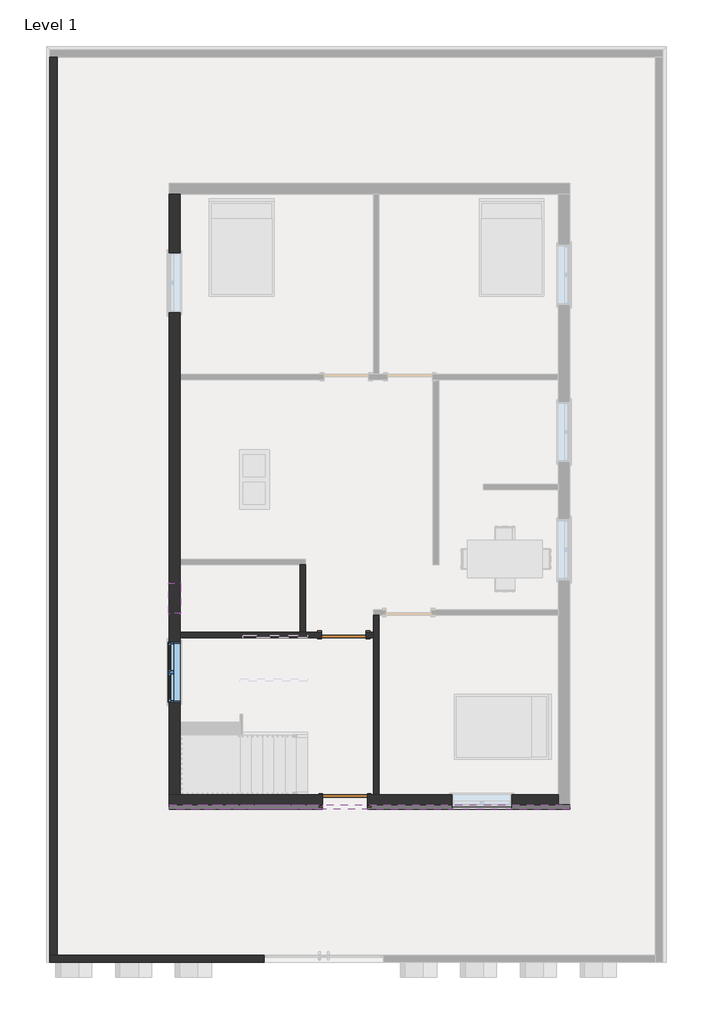
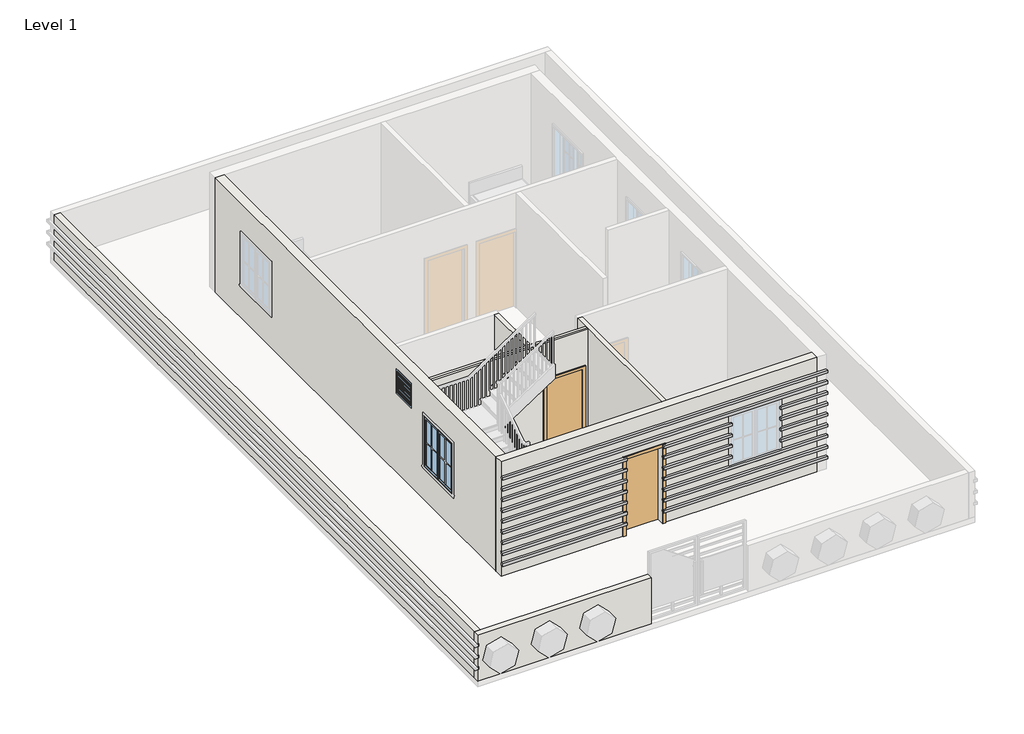
# One storey, part 1 of 4: 9 proxies, 7 walls, 2 doors, 2 windows.
"""IFC4 building model written with IfcOpenShell, lengths in millimetres."""

from ifc_helpers import new_model, si_unit, frame, origin, origin_with_axes, place, context, project, spatial, polyline, outline, extrude, faceted_brep, transform, mapped, element, save
from components import single_flush_door_3_5e62189b, single_flush_door_3_89fc3733, window_casement_double_window_4_576b2d2c, window_f2d8fef0

model = new_model("IFC4")

# Units and contexts
model_context = context("Model", 3, world=origin())
ifc_project = project(units=[si_unit("LENGTHUNIT", "METRE", prefix="MILLI")], contexts=[model_context])

# Site, building, storey
site = spatial("IfcSite", under=ifc_project)
building = spatial("IfcBuilding", under=site)
storey = spatial("IfcBuildingStorey", under=building, Name="Level 1", Elevation=0.0)

# Proxies
placement = place(None, origin())
element("IfcBuildingElementProxy", 1, Name="Reveal", ObjectType="Reveal", at=placement, inside=storey, context=model_context, shape_type="SweptSolid", body=[
    extrude(outline(polyline([(2831.4882597, -6585.4426559), (2831.4882597, -6677.5176559), (-1289.6617403, -6677.5176559), (-1289.6617403, -6585.4426559), (2831.4882597, -6585.4426559)])), frame((0.0, 0.0, 304.8), z_axis=(0.0, 0.0, 1.0), x_axis=(1.0, 0.0, 0.0)), (0.0, 0.0, 1.0), 67.7333333),
    extrude(outline(polyline([(-2204.0617403, -6585.4426559), (-2204.0617403, -6677.5176559), (-5334.6117403, -6677.5176559), (-5334.6117403, -6585.4426559), (-2204.0617403, -6585.4426559)])), frame((0.0, 0.0, 304.8), z_axis=(0.0, 0.0, 1.0), x_axis=(1.0, 0.0, 0.0)), (0.0, 0.0, 1.0), 67.7333333),
])
element("IfcBuildingElementProxy", 2, Name="Reveal", ObjectType="Reveal", at=placement, inside=storey, context=model_context, shape_type="SweptSolid", body=[
    extrude(outline(polyline([(2831.4882597, -6585.4426559), (2831.4882597, -6677.5176559), (-1289.6617403, -6677.5176559), (-1289.6617403, -6585.4426559), (2831.4882597, -6585.4426559)])), frame((0.0, 0.0, 591.2994231), z_axis=(0.0, 0.0, 1.0), x_axis=(1.0, 0.0, 0.0)), (0.0, 0.0, 1.0), 67.7333333),
    extrude(outline(polyline([(-2204.0617403, -6585.4426559), (-2204.0617403, -6677.5176559), (-5334.6117403, -6677.5176559), (-5334.6117403, -6585.4426559), (-2204.0617403, -6585.4426559)])), frame((0.0, 0.0, 591.2994231), z_axis=(0.0, 0.0, 1.0), x_axis=(1.0, 0.0, 0.0)), (0.0, 0.0, 1.0), 67.7333333),
])
element("IfcBuildingElementProxy", 3, Name="Reveal", ObjectType="Reveal", at=placement, inside=storey, context=model_context, shape_type="SweptSolid", body=[
    extrude(outline(polyline([(2831.4882597, -6585.4426559), (2831.4882597, -6677.5176559), (-1289.6617403, -6677.5176559), (-1289.6617403, -6585.4426559), (2831.4882597, -6585.4426559)])), frame((0.0, 0.0, 877.7988461), z_axis=(0.0, 0.0, 1.0), x_axis=(1.0, 0.0, 0.0)), (0.0, 0.0, 1.0), 67.7333333),
    extrude(outline(polyline([(-2204.0617403, -6585.4426559), (-2204.0617403, -6677.5176559), (-5334.6117403, -6677.5176559), (-5334.6117403, -6585.4426559), (-2204.0617403, -6585.4426559)])), frame((0.0, 0.0, 877.7988461), z_axis=(0.0, 0.0, 1.0), x_axis=(1.0, 0.0, 0.0)), (0.0, 0.0, 1.0), 67.7333333),
])
element("IfcBuildingElementProxy", 4, Name="Reveal", ObjectType="Reveal", at=placement, inside=storey, context=model_context, shape_type="SweptSolid", body=[
    extrude(outline(polyline([(2831.4882597, -6585.4426559), (2831.4882597, -6677.5176559), (1650.3882597, -6677.5176559), (1650.3882597, -6585.4426559), (2831.4882597, -6585.4426559)])), frame((0.0, 0.0, 1164.2982692), z_axis=(0.0, 0.0, 1.0), x_axis=(1.0, 0.0, 0.0)), (0.0, 0.0, 1.0), 67.7333333),
    extrude(outline(polyline([(431.1882597, -6585.4426559), (431.1882597, -6677.5176559), (-1289.6617403, -6677.5176559), (-1289.6617403, -6585.4426559), (431.1882597, -6585.4426559)])), frame((0.0, 0.0, 1164.2982692), z_axis=(0.0, 0.0, 1.0), x_axis=(1.0, 0.0, 0.0)), (0.0, 0.0, 1.0), 67.7333333),
    extrude(outline(polyline([(-2204.0617403, -6585.4426559), (-2204.0617403, -6677.5176559), (-5334.6117403, -6677.5176559), (-5334.6117403, -6585.4426559), (-2204.0617403, -6585.4426559)])), frame((0.0, 0.0, 1164.2982692), z_axis=(0.0, 0.0, 1.0), x_axis=(1.0, 0.0, 0.0)), (0.0, 0.0, 1.0), 67.7333333),
])
element("IfcBuildingElementProxy", 5, Name="Reveal", ObjectType="Reveal", at=placement, inside=storey, context=model_context, shape_type="SweptSolid", body=[
    extrude(outline(polyline([(2831.4882597, -6585.4426559), (2831.4882597, -6677.5176559), (1650.3882597, -6677.5176559), (1650.3882597, -6585.4426559), (2831.4882597, -6585.4426559)])), frame((0.0, 0.0, 1450.7976923), z_axis=(0.0, 0.0, 1.0), x_axis=(1.0, 0.0, 0.0)), (0.0, 0.0, 1.0), 67.7333333),
    extrude(outline(polyline([(431.1882597, -6585.4426559), (431.1882597, -6677.5176559), (-1289.6617403, -6677.5176559), (-1289.6617403, -6585.4426559), (431.1882597, -6585.4426559)])), frame((0.0, 0.0, 1450.7976923), z_axis=(0.0, 0.0, 1.0), x_axis=(1.0, 0.0, 0.0)), (0.0, 0.0, 1.0), 67.7333333),
    extrude(outline(polyline([(-2204.0617403, -6585.4426559), (-2204.0617403, -6677.5176559), (-5334.6117403, -6677.5176559), (-5334.6117403, -6585.4426559), (-2204.0617403, -6585.4426559)])), frame((0.0, 0.0, 1450.7976923), z_axis=(0.0, 0.0, 1.0), x_axis=(1.0, 0.0, 0.0)), (0.0, 0.0, 1.0), 67.7333333),
])
element("IfcBuildingElementProxy", 6, Name="Reveal", ObjectType="Reveal", at=placement, inside=storey, context=model_context, shape_type="SweptSolid", body=[
    extrude(outline(polyline([(2831.4882597, -6585.4426559), (2831.4882597, -6677.5176559), (1650.3882597, -6677.5176559), (1650.3882597, -6585.4426559), (2831.4882597, -6585.4426559)])), frame((0.0, 0.0, 1737.2971154), z_axis=(0.0, 0.0, 1.0), x_axis=(1.0, 0.0, 0.0)), (0.0, 0.0, 1.0), 67.7333333),
    extrude(outline(polyline([(431.1882597, -6585.4426559), (431.1882597, -6677.5176559), (-1289.6617403, -6677.5176559), (-1289.6617403, -6585.4426559), (431.1882597, -6585.4426559)])), frame((0.0, 0.0, 1737.2971154), z_axis=(0.0, 0.0, 1.0), x_axis=(1.0, 0.0, 0.0)), (0.0, 0.0, 1.0), 67.7333333),
    extrude(outline(polyline([(-2204.0617403, -6585.4426559), (-2204.0617403, -6677.5176559), (-5334.6117403, -6677.5176559), (-5334.6117403, -6585.4426559), (-2204.0617403, -6585.4426559)])), frame((0.0, 0.0, 1737.2971154), z_axis=(0.0, 0.0, 1.0), x_axis=(1.0, 0.0, 0.0)), (0.0, 0.0, 1.0), 67.7333333),
])
element("IfcBuildingElementProxy", 7, Name="Reveal", ObjectType="Reveal", at=placement, inside=storey, context=model_context, shape_type="SweptSolid", body=[
    extrude(outline(polyline([(2831.4882597, -6585.4426559), (2831.4882597, -6677.5176559), (1650.3882597, -6677.5176559), (1650.3882597, -6585.4426559), (2831.4882597, -6585.4426559)])), frame((0.0, 0.0, 2023.7965384), z_axis=(0.0, 0.0, 1.0), x_axis=(1.0, 0.0, 0.0)), (0.0, 0.0, 1.0), 67.7333333),
    extrude(outline(polyline([(431.1882597, -6585.4426559), (431.1882597, -6677.5176559), (-1289.6617403, -6677.5176559), (-1289.6617403, -6585.4426559), (431.1882597, -6585.4426559)])), frame((0.0, 0.0, 2023.7965384), z_axis=(0.0, 0.0, 1.0), x_axis=(1.0, 0.0, 0.0)), (0.0, 0.0, 1.0), 67.7333333),
    extrude(outline(polyline([(-2204.0617403, -6585.4426559), (-2204.0617403, -6677.5176559), (-5334.6117403, -6677.5176559), (-5334.6117403, -6585.4426559), (-2204.0617403, -6585.4426559)])), frame((0.0, 0.0, 2023.7965384), z_axis=(0.0, 0.0, 1.0), x_axis=(1.0, 0.0, 0.0)), (0.0, 0.0, 1.0), 67.7333333),
])
element("IfcBuildingElementProxy", 8, Name="Reveal", ObjectType="Reveal", at=placement, inside=storey, context=model_context, shape_type="SweptSolid", body=[
    extrude(outline(polyline([(2831.4882597, -6585.4426559), (2831.4882597, -6677.5176559), (-5334.6117403, -6677.5176559), (-5334.6117403, -6585.4426559), (2831.4882597, -6585.4426559)])), frame((0.0, 0.0, 2310.2959615), z_axis=(0.0, 0.0, 1.0), x_axis=(1.0, 0.0, 0.0)), (0.0, 0.0, 1.0), 67.7333333),
])
element("IfcBuildingElementProxy", 9, Name="Reveal", ObjectType="Reveal", at=placement, inside=storey, context=model_context, shape_type="SweptSolid", body=[
    extrude(outline(polyline([(2831.4882597, -6585.4426559), (2831.4882597, -6677.5176559), (-5334.6117403, -6677.5176559), (-5334.6117403, -6585.4426559), (2831.4882597, -6585.4426559)])), frame((0.0, 0.0, 2596.7953846), z_axis=(0.0, 0.0, 1.0), x_axis=(1.0, 0.0, 0.0)), (0.0, 0.0, 1.0), 67.7333333),
])

# Doors
single_flush_door_3_shape = single_flush_door_3_5e62189b(model_context)
element("IfcDoor", 10, ObjectType="Single-Flush : DOOR 3'", at=placement, inside=storey, context=model_context, shape_type="MappedRepresentation", body=[
    mapped(single_flush_door_3_shape, transform((-1772.2617403, -3124.6926559, 0.0), x_axis=(1.0, 0.0, 0.0), y_axis=(0.0, 1.0, 0.0), z_axis=(0.0, 0.0, 1.0))),
])
single_flush_door_3_2_shape = single_flush_door_3_89fc3733(model_context)
element("IfcDoor", 11, ObjectType="Single-Flush : DOOR 3'", at=placement, inside=storey, context=model_context, shape_type="MappedRepresentation", body=[
    mapped(single_flush_door_3_2_shape, transform((-1746.8617403, -6496.5426559, 0.0), x_axis=(1.0, 0.0, 0.0), y_axis=(0.0, 1.0, 0.0), z_axis=(0.0, 0.0, 1.0))),
])

# Walls
element("IfcWall", 12, ObjectType="ALL 4.5\"", at=placement, inside=storey, context=model_context, shape_type="Brep", body=[
    faceted_brep([(-1169.0117403, -2724.6426559, 0.0), (-1169.0117403, -3067.5426559, 0.0), (-1169.0117403, -3181.8426559, 0.0), (-1169.0117403, -6382.2426559, 0.0), (-1169.0117403, -6382.2426559, 3048.0), (-1169.0117403, -3181.8426559, 3048.0), (-1169.0117403, -3067.5426559, 3048.0), (-1169.0117403, -2724.6426559, 3048.0), (-1054.7117403, -2724.6426559, 0.0), (-1054.7117403, -2724.6426559, 3048.0), (-1054.7117403, -6382.2426559, 3048.0), (-1054.7117403, -6382.2426559, 0.0)], [[[0, 1, 2, 3, 4, 5, 6, 7]], [[8, 9, 10, 11]], [[3, 2, 1, 0, 8, 11]], [[0, 7, 9, 8]], [[4, 3, 11, 10]], [[7, 6, 5, 4, 10, 9]]]),
])
element("IfcWall", 13, ObjectType="ALL 4.5\"", at=placement, inside=storey, context=model_context, shape_type="Brep", body=[
    faceted_brep([(-1169.0117403, -3067.5426559, 0.0), (-1315.0617403, -3067.5426559, 0.0), (-1315.0617403, -3067.5426559, 2032.0), (-2229.4617403, -3067.5426559, 2032.0), (-2229.4617403, -3067.5426559, 0.0), (-2553.3117403, -3067.5426559, 0.0), (-2667.6117403, -3067.5426559, 0.0), (-5106.0117403, -3067.5426559, 0.0), (-5106.0117403, -3067.5426559, 3048.0), (-2667.6117403, -3067.5426559, 3048.0), (-2553.3117403, -3067.5426559, 3048.0), (-1169.0117403, -3067.5426559, 3048.0), (-1315.0617403, -3181.8426559, 2032.0), (-1315.0617403, -3181.8426559, 0.0), (-1169.0117403, -3181.8426559, 0.0), (-1169.0117403, -3181.8426559, 3048.0), (-5106.0117403, -3181.8426559, 3048.0), (-5106.0117403, -3181.8426559, 0.0), (-2229.4617403, -3181.8426559, 0.0), (-2229.4617403, -3181.8426559, 2032.0), (-5106.0117403, -3131.0426559, 3048.0), (-1169.0117403, -3131.0426559, 3048.0), (-2515.2117403, -3131.0426559, 3048.0)], [[[0, 1, 2, 3, 4, 5, 6, 7, 8, 9, 10, 11]], [[12, 13, 14, 15, 16, 17, 18, 19]], [[18, 17, 7, 6, 5, 4]], [[14, 13, 1, 0]], [[8, 7, 17, 16, 20]], [[0, 11, 21, 15, 14]], [[2, 1, 13, 12]], [[3, 2, 12, 19]], [[4, 3, 19, 18]], [[11, 10, 9, 8, 20, 22, 21]], [[20, 16, 15, 21, 22]]]),
])
element("IfcWall", 14, ObjectType="ALL 4.5\"", at=placement, inside=storey, context=model_context, shape_type="SweptSolid", body=[
    extrude(outline(polyline([(-2667.6117403, -3067.5426559), (-2667.6117403, -1695.9426559), (-2553.3117403, -1695.9426559), (-2553.3117403, -3067.5426559), (-2667.6117403, -3067.5426559)])), origin_with_axes(), (0.0, 0.0, 1.0), 3048.0),
])
element("IfcWall", 15, ObjectType="CMD 6\"", at=placement, inside=storey, context=model_context, shape_type="SweptSolid", body=[
    extrude(outline(polyline([(0.0, -7613.2753152), (1219.2, -7613.2753152), (1219.2, -7765.6753152), (982.1333333, -7765.6753152), (982.1333333, -7740.2753152), (914.4, -7740.2753152), (914.4, -7765.6753152), (677.3333333, -7765.6753152), (677.3333333, -7740.2753152), (609.6, -7740.2753152), (609.6, -7765.6753152), (372.5333333, -7765.6753152), (372.5333333, -7740.2753152), (304.8, -7740.2753152), (304.8, -7765.6753152), (0.0, -7765.6753152), (0.0, -7613.2753152)])), frame((0.0, -9645.3989753, 0.0), z_axis=(0.0, 1.0, 0.0), x_axis=(0.0, 0.0, 1.0)), (0.0, 0.0, 1.0), 18288.0),
])
element("IfcWall", 16, ObjectType="CMD 6\"", at=placement, inside=storey, context=model_context, shape_type="Brep", body=[
    faceted_brep([(-3397.8617403, -9645.3989753, 0.0), (-7613.2753152, -9645.3989753, 0.0), (-7765.6753152, -9645.3989753, 0.0), (-7765.6753152, -9645.3989753, 304.8), (-7740.2753152, -9645.3989753, 304.8), (-7740.2753152, -9645.3989753, 372.5333333), (-7765.6753152, -9645.3989753, 372.5333333), (-7765.6753152, -9645.3989753, 609.6), (-7740.2753152, -9645.3989753, 609.6), (-7740.2753152, -9645.3989753, 677.3333333), (-7765.6753152, -9645.3989753, 677.3333333), (-7765.6753152, -9645.3989753, 914.4), (-7740.2753152, -9645.3989753, 914.4), (-7740.2753152, -9645.3989753, 982.1333333), (-7765.6753152, -9645.3989753, 982.1333333), (-7765.6753152, -9645.3989753, 1219.2), (-7613.2753152, -9645.3989753, 1219.2), (-3397.8617403, -9645.3989753, 1219.2), (-7765.6753152, -9797.7989753, 0.0), (-3397.8617403, -9797.7989753, 0.0), (-3397.8617403, -9797.7989753, 1219.2), (-7765.6753152, -9797.7989753, 1219.2), (-7765.6753152, -9797.7989753, 982.1333333), (-7740.2753152, -9797.7989753, 982.1333333), (-7740.2753152, -9797.7989753, 914.4), (-7765.6753152, -9797.7989753, 914.4), (-7765.6753152, -9797.7989753, 677.3333333), (-7740.2753152, -9797.7989753, 677.3333333), (-7740.2753152, -9797.7989753, 609.6), (-7765.6753152, -9797.7989753, 609.6), (-7765.6753152, -9797.7989753, 372.5333333), (-7740.2753152, -9797.7989753, 372.5333333), (-7740.2753152, -9797.7989753, 304.8), (-7765.6753152, -9797.7989753, 304.8)], [[[0, 1, 2, 3, 4, 5, 6, 7, 8, 9, 10, 11, 12, 13, 14, 15, 16, 17]], [[18, 19, 20, 21, 22, 23, 24, 25, 26, 27, 28, 29, 30, 31, 32, 33]], [[2, 1, 0, 19, 18]], [[17, 16, 15, 21, 20]], [[0, 17, 20, 19]], [[2, 18, 33, 3]], [[21, 15, 14, 22]], [[6, 30, 29, 7]], [[10, 26, 25, 11]], [[5, 31, 30, 6]], [[32, 4, 3, 33]], [[31, 5, 4, 32]], [[9, 27, 26, 10]], [[28, 8, 7, 29]], [[27, 9, 8, 28]], [[13, 23, 22, 14]], [[24, 12, 11, 25]], [[23, 13, 12, 24]]]),
])
element("IfcWall", 17, ObjectType="WALL 9\"", at=placement, inside=storey, context=model_context, shape_type="Brep", body=[
    faceted_brep([(-5334.6117403, -6382.2426559, 3048.0), (-5106.0117403, -6382.2426559, 3048.0), (-1169.0117403, -6382.2426559, 3048.0), (-1054.7117403, -6382.2426559, 3048.0), (2602.8882597, -6382.2426559, 3048.0), (2602.8882597, -6382.2426559, 0.0), (-1054.7117403, -6382.2426559, 0.0), (-1169.0117403, -6382.2426559, 0.0), (-1289.6617403, -6382.2426559, 0.0), (-1289.6617403, -6382.2426559, 2032.0), (-2204.0617403, -6382.2426559, 2032.0), (-2204.0617403, -6382.2426559, 0.0), (-5106.0117403, -6382.2426559, 0.0), (-5334.6117403, -6382.2426559, 0.0), (431.1882597, -6382.2426559, 2260.6), (431.1882597, -6382.2426559, 914.4), (1650.3882597, -6382.2426559, 914.4), (1650.3882597, -6382.2426559, 2260.6), (2602.8882597, -6610.8426559, 3048.0), (-5334.6117403, -6610.8426559, 3048.0), (-5334.6117403, -6610.8426559, 2664.5287179), (2602.8882597, -6610.8426559, 2664.5287179), (431.1882597, -6610.8426559, 2260.6), (1650.3882597, -6610.8426559, 2260.6), (1650.3882597, -6610.8426559, 2091.5298718), (2602.8882597, -6610.8426559, 2091.5298718), (2602.8882597, -6610.8426559, 2310.2959615), (-5334.6117403, -6610.8426559, 2310.2959615), (-5334.6117403, -6610.8426559, 2091.5298718), (-2204.0617403, -6610.8426559, 2091.5298718), (-2204.0617403, -6610.8426559, 2032.0), (-1289.6617403, -6610.8426559, 2032.0), (-1289.6617403, -6610.8426559, 2091.5298718), (431.1882597, -6610.8426559, 2091.5298718), (-5334.6117403, -6610.8426559, 0.0), (-2204.0617403, -6610.8426559, 0.0), (-2204.0617403, -6610.8426559, 304.8), (-5334.6117403, -6610.8426559, 304.8), (-1289.6617403, -6610.8426559, 0.0), (2602.8882597, -6610.8426559, 0.0), (2602.8882597, -6610.8426559, 304.8), (-1289.6617403, -6610.8426559, 304.8), (-1289.6617403, -6610.8426559, 372.5333333), (2602.8882597, -6610.8426559, 372.5333333), (2602.8882597, -6610.8426559, 591.2994231), (-1289.6617403, -6610.8426559, 591.2994231), (-5334.6117403, -6610.8426559, 372.5333333), (-2204.0617403, -6610.8426559, 372.5333333), (-2204.0617403, -6610.8426559, 591.2994231), (-5334.6117403, -6610.8426559, 591.2994231), (-1289.6617403, -6610.8426559, 659.0327564), (2602.8882597, -6610.8426559, 659.0327564), (2602.8882597, -6610.8426559, 877.7988461), (-1289.6617403, -6610.8426559, 877.7988461), (-5334.6117403, -6610.8426559, 659.0327564), (-2204.0617403, -6610.8426559, 659.0327564), (-2204.0617403, -6610.8426559, 877.7988461), (-5334.6117403, -6610.8426559, 877.7988461), (-1289.6617403, -6610.8426559, 945.5321795), (431.1882597, -6610.8426559, 945.5321795), (431.1882597, -6610.8426559, 1164.2982692), (-1289.6617403, -6610.8426559, 1164.2982692), (1650.3882597, -6610.8426559, 945.5321795), (2602.8882597, -6610.8426559, 945.5321795), (2602.8882597, -6610.8426559, 1164.2982692), (1650.3882597, -6610.8426559, 1164.2982692), (-5334.6117403, -6610.8426559, 945.5321795), (-2204.0617403, -6610.8426559, 945.5321795), (-2204.0617403, -6610.8426559, 1164.2982692), (-5334.6117403, -6610.8426559, 1164.2982692), (1650.3882597, -6610.8426559, 1232.0316025), (2602.8882597, -6610.8426559, 1232.0316025), (2602.8882597, -6610.8426559, 1450.7976923), (1650.3882597, -6610.8426559, 1450.7976923), (-1289.6617403, -6610.8426559, 1232.0316025), (431.1882597, -6610.8426559, 1232.0316025), (431.1882597, -6610.8426559, 1450.7976923), (-1289.6617403, -6610.8426559, 1450.7976923), (-5334.6117403, -6610.8426559, 1232.0316025), (-2204.0617403, -6610.8426559, 1232.0316025), (-2204.0617403, -6610.8426559, 1450.7976923), (-5334.6117403, -6610.8426559, 1450.7976923), (1650.3882597, -6610.8426559, 1518.5310256), (2602.8882597, -6610.8426559, 1518.5310256), (2602.8882597, -6610.8426559, 1737.2971154), (1650.3882597, -6610.8426559, 1737.2971154), (-1289.6617403, -6610.8426559, 1518.5310256), (431.1882597, -6610.8426559, 1518.5310256), (431.1882597, -6610.8426559, 1737.2971154), (-1289.6617403, -6610.8426559, 1737.2971154), (-5334.6117403, -6610.8426559, 1518.5310256), (-2204.0617403, -6610.8426559, 1518.5310256), (-2204.0617403, -6610.8426559, 1737.2971154), (-5334.6117403, -6610.8426559, 1737.2971154), (1650.3882597, -6610.8426559, 1805.0304487), (2602.8882597, -6610.8426559, 1805.0304487), (2602.8882597, -6610.8426559, 2023.7965384), (1650.3882597, -6610.8426559, 2023.7965384), (-1289.6617403, -6610.8426559, 1805.0304487), (431.1882597, -6610.8426559, 1805.0304487), (431.1882597, -6610.8426559, 2023.7965384), (-1289.6617403, -6610.8426559, 2023.7965384), (-5334.6117403, -6610.8426559, 1805.0304487), (-2204.0617403, -6610.8426559, 1805.0304487), (-2204.0617403, -6610.8426559, 2023.7965384), (-5334.6117403, -6610.8426559, 2023.7965384), (-5334.6117403, -6610.8426559, 2378.0292948), (2602.8882597, -6610.8426559, 2378.0292948), (2602.8882597, -6610.8426559, 2596.7953846), (-5334.6117403, -6610.8426559, 2596.7953846), (2602.8882597, -6585.4426559, 2664.5287179), (2602.8882597, -6585.4426559, 2596.7953846), (2602.8882597, -6585.4426559, 2378.0292948), (2602.8882597, -6585.4426559, 2310.2959615), (2602.8882597, -6585.4426559, 2091.5298718), (2602.8882597, -6585.4426559, 2023.7965384), (2602.8882597, -6585.4426559, 1805.0304487), (2602.8882597, -6585.4426559, 1737.2971154), (2602.8882597, -6585.4426559, 1518.5310256), (2602.8882597, -6585.4426559, 1450.7976923), (2602.8882597, -6585.4426559, 1232.0316025), (2602.8882597, -6585.4426559, 1164.2982692), (2602.8882597, -6585.4426559, 945.5321795), (2602.8882597, -6585.4426559, 877.7988461), (2602.8882597, -6585.4426559, 659.0327564), (2602.8882597, -6585.4426559, 591.2994231), (2602.8882597, -6585.4426559, 372.5333333), (2602.8882597, -6585.4426559, 304.8), (-5334.6117403, -6585.4426559, 304.8), (-5334.6117403, -6585.4426559, 372.5333333), (-5334.6117403, -6585.4426559, 591.2994231), (-5334.6117403, -6585.4426559, 659.0327564), (-5334.6117403, -6585.4426559, 877.7988461), (-5334.6117403, -6585.4426559, 945.5321795), (-5334.6117403, -6585.4426559, 1164.2982692), (-5334.6117403, -6585.4426559, 1232.0316025), (-5334.6117403, -6585.4426559, 1450.7976923), (-5334.6117403, -6585.4426559, 1518.5310256), (-5334.6117403, -6585.4426559, 1737.2971154), (-5334.6117403, -6585.4426559, 1805.0304487), (-5334.6117403, -6585.4426559, 2023.7965384), (-5334.6117403, -6585.4426559, 2091.5298718), (-5334.6117403, -6585.4426559, 2310.2959615), (-5334.6117403, -6585.4426559, 2378.0292948), (-5334.6117403, -6585.4426559, 2596.7953846), (-5334.6117403, -6585.4426559, 2664.5287179), (431.1882597, -6585.4426559, 2091.5298718), (431.1882597, -6585.4426559, 2023.7965384), (431.1882597, -6585.4426559, 1805.0304487), (431.1882597, -6585.4426559, 1737.2971154), (431.1882597, -6585.4426559, 1518.5310256), (431.1882597, -6585.4426559, 1450.7976923), (431.1882597, -6585.4426559, 1232.0316025), (431.1882597, -6585.4426559, 1164.2982692), (431.1882597, -6585.4426559, 945.5321795), (431.1882597, -6585.4426559, 914.4), (1650.3882597, -6585.4426559, 914.4), (1650.3882597, -6585.4426559, 945.5321795), (1650.3882597, -6585.4426559, 1164.2982692), (1650.3882597, -6585.4426559, 1232.0316025), (1650.3882597, -6585.4426559, 1450.7976923), (1650.3882597, -6585.4426559, 1518.5310256), (1650.3882597, -6585.4426559, 1737.2971154), (1650.3882597, -6585.4426559, 1805.0304487), (1650.3882597, -6585.4426559, 2023.7965384), (1650.3882597, -6585.4426559, 2091.5298718), (-1289.6617403, -6585.4426559, 304.8), (-1289.6617403, -6585.4426559, 372.5333333), (-1289.6617403, -6585.4426559, 591.2994231), (-1289.6617403, -6585.4426559, 659.0327564), (-1289.6617403, -6585.4426559, 877.7988461), (-1289.6617403, -6585.4426559, 945.5321795), (-1289.6617403, -6585.4426559, 1164.2982692), (-1289.6617403, -6585.4426559, 1232.0316025), (-1289.6617403, -6585.4426559, 1450.7976923), (-1289.6617403, -6585.4426559, 1518.5310256), (-1289.6617403, -6585.4426559, 1737.2971154), (-1289.6617403, -6585.4426559, 1805.0304487), (-1289.6617403, -6585.4426559, 2023.7965384), (-1289.6617403, -6585.4426559, 2032.0), (-2204.0617403, -6585.4426559, 2032.0), (-2204.0617403, -6585.4426559, 2023.7965384), (-2204.0617403, -6585.4426559, 1805.0304487), (-2204.0617403, -6585.4426559, 1737.2971154), (-2204.0617403, -6585.4426559, 1518.5310256), (-2204.0617403, -6585.4426559, 1450.7976923), (-2204.0617403, -6585.4426559, 1232.0316025), (-2204.0617403, -6585.4426559, 1164.2982692), (-2204.0617403, -6585.4426559, 945.5321795), (-2204.0617403, -6585.4426559, 877.7988461), (-2204.0617403, -6585.4426559, 659.0327564), (-2204.0617403, -6585.4426559, 591.2994231), (-2204.0617403, -6585.4426559, 372.5333333), (-2204.0617403, -6585.4426559, 304.8), (-1289.6617403, -6585.4426559, 2091.5298718), (-2204.0617403, -6585.4426559, 2091.5298718)], [[[0, 1, 2, 3, 4, 5, 6, 7, 8, 9, 10, 11, 12, 13], [14, 15, 16, 17]], [[18, 19, 20, 21]], [[22, 23, 24, 25, 26, 27, 28, 29, 30, 31, 32, 33]], [[34, 35, 36, 37]], [[38, 39, 40, 41]], [[42, 43, 44, 45]], [[46, 47, 48, 49]], [[50, 51, 52, 53]], [[54, 55, 56, 57]], [[58, 59, 60, 61]], [[62, 63, 64, 65]], [[66, 67, 68, 69]], [[70, 71, 72, 73]], [[74, 75, 76, 77]], [[78, 79, 80, 81]], [[82, 83, 84, 85]], [[86, 87, 88, 89]], [[90, 91, 92, 93]], [[94, 95, 96, 97]], [[98, 99, 100, 101]], [[102, 103, 104, 105]], [[106, 107, 108, 109]], [[5, 39, 38, 8, 7, 6]], [[34, 13, 12, 11, 35]], [[4, 3, 2, 1, 0, 19, 18]], [[5, 4, 18, 21, 110, 111, 108, 107, 112, 113, 26, 25, 114, 115, 96, 95, 116, 117, 84, 83, 118, 119, 72, 71, 120, 121, 64, 63, 122, 123, 52, 51, 124, 125, 44, 43, 126, 127, 40, 39]], [[0, 13, 34, 37, 128, 129, 46, 49, 130, 131, 54, 57, 132, 133, 66, 69, 134, 135, 78, 81, 136, 137, 90, 93, 138, 139, 102, 105, 140, 141, 28, 27, 142, 143, 106, 109, 144, 145, 20, 19]], [[15, 14, 22, 33, 146, 147, 100, 99, 148, 149, 88, 87, 150, 151, 76, 75, 152, 153, 60, 59, 154, 155]], [[16, 15, 155, 156]], [[17, 16, 156, 157, 62, 65, 158, 159, 70, 73, 160, 161, 82, 85, 162, 163, 94, 97, 164, 165, 24, 23]], [[14, 17, 23, 22]], [[9, 8, 38, 41, 166, 167, 42, 45, 168, 169, 50, 53, 170, 171, 58, 61, 172, 173, 74, 77, 174, 175, 86, 89, 176, 177, 98, 101, 178, 179]], [[10, 9, 179, 31, 30, 180]], [[11, 10, 180, 181, 104, 103, 182, 183, 92, 91, 184, 185, 80, 79, 186, 187, 68, 67, 188, 189, 56, 55, 190, 191, 48, 47, 192, 193, 36, 35]], [[167, 126, 43, 42]], [[127, 166, 41, 40]], [[126, 167, 166, 127]], [[129, 192, 47, 46]], [[193, 128, 37, 36]], [[192, 129, 128, 193]], [[169, 124, 51, 50]], [[125, 168, 45, 44]], [[124, 169, 168, 125]], [[131, 190, 55, 54]], [[191, 130, 49, 48]], [[190, 131, 130, 191]], [[171, 154, 59, 58]], [[157, 122, 63, 62]], [[123, 170, 53, 52]], [[154, 171, 170, 123, 122, 157, 156, 155]], [[133, 188, 67, 66]], [[189, 132, 57, 56]], [[188, 133, 132, 189]], [[159, 120, 71, 70]], [[121, 158, 65, 64]], [[120, 159, 158, 121]], [[173, 152, 75, 74]], [[153, 172, 61, 60]], [[152, 173, 172, 153]], [[135, 186, 79, 78]], [[187, 134, 69, 68]], [[186, 135, 134, 187]], [[161, 118, 83, 82]], [[119, 160, 73, 72]], [[118, 161, 160, 119]], [[175, 150, 87, 86]], [[151, 174, 77, 76]], [[150, 175, 174, 151]], [[137, 184, 91, 90]], [[185, 136, 81, 80]], [[184, 137, 136, 185]], [[163, 116, 95, 94]], [[117, 162, 85, 84]], [[116, 163, 162, 117]], [[177, 148, 99, 98]], [[149, 176, 89, 88]], [[148, 177, 176, 149]], [[139, 182, 103, 102]], [[183, 138, 93, 92]], [[182, 139, 138, 183]], [[165, 114, 25, 24]], [[115, 164, 97, 96]], [[114, 165, 164, 115]], [[179, 194, 32, 31]], [[194, 146, 33, 32]], [[147, 178, 101, 100]], [[146, 194, 179, 178, 147]], [[195, 180, 30, 29]], [[141, 195, 29, 28]], [[181, 140, 105, 104]], [[195, 141, 140, 181, 180]], [[143, 112, 107, 106]], [[113, 142, 27, 26]], [[112, 143, 142, 113]], [[145, 110, 21, 20]], [[111, 144, 109, 108]], [[110, 145, 144, 111]]]),
])
element("IfcWall", 18, ObjectType="WALL 9\"", at=placement, inside=storey, context=model_context, shape_type="Brep", body=[
    faceted_brep([(-5106.0117403, -6382.2426559, 0.0), (-5106.0117403, -3181.8426559, 0.0), (-5106.0117403, -3067.5426559, 0.0), (-5106.0117403, -1695.9426559, 0.0), (-5106.0117403, -1581.6426559, 0.0), (-5106.0117403, 2075.9573441, 0.0), (-5106.0117403, 2190.2573441, 0.0), (-5106.0117403, 5847.8573441, 0.0), (-5106.0117403, 5847.8573441, 3048.0), (-5106.0117403, 2190.2573441, 3048.0), (-5106.0117403, 2075.9573441, 3048.0), (-5106.0117403, -1581.6426559, 3048.0), (-5106.0117403, -1695.9426559, 3048.0), (-5106.0117403, -3067.5426559, 3048.0), (-5106.0117403, -3181.8426559, 3048.0), (-5106.0117403, -6382.2426559, 3048.0), (-5106.0117403, -3277.0926559, 2260.6), (-5106.0117403, -3277.0926559, 914.4), (-5106.0117403, -4496.2926559, 914.4), (-5106.0117403, -4496.2926559, 2260.6), (-5106.0117403, 4657.2323441, 2260.6), (-5106.0117403, 4657.2323441, 914.4), (-5106.0117403, 3438.0323441, 914.4), (-5106.0117403, 3438.0323441, 2260.6), (-5106.0117403, -2686.5426559, 2743.2), (-5106.0117403, -2076.9426559, 2743.2), (-5106.0117403, -2076.9426559, 2133.6), (-5106.0117403, -2686.5426559, 2133.6), (-5334.6117403, -6382.2426559, 0.0), (-5334.6117403, -6382.2426559, 3048.0), (-5334.6117403, 5847.8573441, 3048.0), (-5334.6117403, 5847.8573441, 0.0), (-5334.6117403, -3277.0926559, 2260.6), (-5334.6117403, -4496.2926559, 2260.6), (-5334.6117403, -4496.2926559, 914.4), (-5334.6117403, -3277.0926559, 914.4), (-5334.6117403, 4657.2323441, 2260.6), (-5334.6117403, 3438.0323441, 2260.6), (-5334.6117403, 3438.0323441, 914.4), (-5334.6117403, 4657.2323441, 914.4), (-5334.6117403, -2686.5426559, 2743.2), (-5334.6117403, -2686.5426559, 2133.6), (-5334.6117403, -2076.9426559, 2133.6), (-5334.6117403, -2076.9426559, 2743.2)], [[[0, 1, 2, 3, 4, 5, 6, 7, 8, 9, 10, 11, 12, 13, 14, 15], [16, 17, 18, 19], [20, 21, 22, 23], [24, 25, 26, 27]], [[28, 29, 30, 31], [32, 33, 34, 35], [36, 37, 38, 39], [40, 41, 42, 43]], [[7, 6, 5, 4, 3, 2, 1, 0, 28, 31]], [[15, 14, 13, 12, 11, 10, 9, 8, 30, 29]], [[8, 7, 31, 30]], [[0, 15, 29, 28]], [[17, 16, 32, 35]], [[18, 17, 35, 34]], [[19, 18, 34, 33]], [[16, 19, 33, 32]], [[21, 20, 36, 39]], [[22, 21, 39, 38]], [[23, 22, 38, 37]], [[20, 23, 37, 36]], [[41, 40, 24, 27]], [[42, 41, 27, 26]], [[43, 42, 26, 25]], [[40, 43, 25, 24]]]),
])

# Windows
window_casement_double_window_4_shape = window_casement_double_window_4_576b2d2c(model_context)
element("IfcWindow", 19, ObjectType="Window-Casement-Double : WINDOW 4'", at=placement, inside=storey, context=model_context, shape_type="MappedRepresentation", body=[
    mapped(window_casement_double_window_4_shape, transform((-5220.3117403, -3886.6926559, 0.0), x_axis=(0.0, 1.0, 0.0), y_axis=(-1.0, 0.0, 0.0), z_axis=(0.0, 0.0, 1.0))),
])
window_shape = window_f2d8fef0(model_context)
element("IfcWindow", 20, ObjectType="Window-Louvers : 24\" x 24\"", at=placement, inside=storey, context=model_context, shape_type="MappedRepresentation", body=[
    mapped(window_shape, transform((-5226.6617403, -2381.7426559, 1219.2), x_axis=(0.0, 1.0, 0.0), y_axis=(-1.0, 0.0, 0.0), z_axis=(0.0, 0.0, 1.0))),
])

save(model, "model.ifc")

# Revit data of these elements
# Type "Single-Flush : DOOR 3'"
#   Type Mark = "8"
#   Construction Type Id = "MDOOR"
#   Assembly Code = "C1020"
#   Analytic Construction = "Metal"
#   Thickness = 0' - 2"
#   Heat Transfer Coefficient (U) = 0.651978 BTU/(h·ft²·°F)
#   Height = 6' - 8"
#   Trim Projection Ext = 0' - 1"
#   Trim Projection Int = 0' - 1"
#   Trim Width = 0' - 3"
#   Width = 3' - 0"
#   Define Thermal Properties by = 1
#   Door Material = Door - Panel
#   Frame Material = Door - Frame
#   Visual Light Transmittance = 0
#   Solar Heat Gain Coefficient = 0
#   Function = (empty or 0)
#   Wall Closure = (empty or 0)
# Type "ALL 4.5\""
#   Assembly Code = "B2010"
#   Layers, outside or top first: 0' - 4 1/2" no material (function 1)
# Type "CMD 6\""
#   Assembly Code = "B2010"
#   Layers, outside or top first: 0' - 6" "Carpet (1)" (function 1)
# Type "WALL 9\""
#   Assembly Code = "B2010"
#   Layers, outside or top first: 0' - 9" "Carpet (1)" (function 1)
# Type "Window-Casement-Double : WINDOW 4'"
#   Type Mark = "18"
#   Fire Rating = "0.5h"
#   Assembly Code = "B2020100"
#   Analytic Construction = "Double glazing - domestic"
#   Frame Extension [instance default] = 0' - 0 1/4"
#   Window Inset [instance default] = 0' - 0"
#   Wall Thickness [instance default] = 0' - 6"
#   Interior Wall Closure [instance default] = 0' - 2 1/4"
#   Half Width = 2' - 0"
#   Visual Light Transmittance = 0.81
#   Thermal Resistance (R) = 1.8146 (h·ft²·°F)/BTU
#   Solar Heat Gain Coefficient = 0.76
#   Rough Width = 4' - 0 1/2"
#   Rough Height = 4' - 5 1/2"
#   Height = 4' - 5"
#   Heat Transfer Coefficient (U) = 0.5511 BTU/(h·ft²·°F)
#   Exterior Wall Closure [instance default] = 0' - 1 1/4"
#   Extension Jamb [instance default] = 0' - 2 1/4"
#   Default Sill Height = 3' - 0"
#   Width = 4' - 0"
#   Muntin Visibility = yes
#   Interior Trim Visibility [instance default] = yes
#   Exterior Trim Visibility [instance default] = yes
#   Extension Jamb Visibility [instance default] = yes
#   Interior Trim Material = Wood - Stained
#   Muntin Pattern = Muntin Pattern_2x2 : Muntin Pattern_2x2
#   Interior Trim = Trim-Window-Interior-Flat : Picture Frame
#   Interior Frame Material = Wood - Stained
#   Glass Panel Material = Glass
#   Exterior Trim Material = Clad - White
#   Exterior Trim = Trim-Window-Exterior-Flat : with Sill
#   Exterior Frame Material = Clad - White
#   Wall Closure = (empty or 0)
# Type "Window-Louvers : 24\" x 24\""
#   Type Mark = "19"
#   Construction Type Id = "GSP4R"
#   Assembly Code = "B20"
#   Analytic Construction = "1/8 in Pilkington single glazing"
#   Visual Light Transmittance = 0.9
#   Thermal Resistance (R) = 1.53941 (h·ft²·°F)/BTU
#   Solar Heat Gain Coefficient = 0.78
#   Max Height = 1' - 11.74264"
#   Height = 2' - 0"
#   Heat Transfer Coefficient (U) = 0.6496 BTU/(h·ft²·°F)
#   Blade Width [instance default] = 1' - 10 1/2"
#   Blade Vertical Thickness = 0' - 0.35355"
#   Blade Thickness = 0' - 0 1/4"
#   Blade Spacing = 0' - 1 1/2"
#   Blade Height = 0' - 1.85355"
#   Blade Depth = 0' - 3"
#   Blade Angle = 45.00°
#   Default Sill Height = 3' - 0"
#   Trim Projection_Exterior = 0' - 0 1/2"
#   Trim Projection_Interior = 0' - 0 1/2"
#   Trim Width_Exterior = 0' - 1 1/2"
#   Trim Width_Interior = 0' - 1 1/2"
#   Width = 2' - 0"
#   Max Blade Count = 12
#   Define Thermal Properties by = 1
#   Blade Count = 12
#   Frame Material = Birch
#   Louver Material = Birch
#   Trim Exterior Material = Birch
#   Trim Interior Material = Birch
#   Wall Closure = (empty or 0)
# Elements 10, 11 (IfcDoor, "Single-Flush : DOOR 3'")
#   Phase Created = New Construction
#   Materials on its faces: "Door - Frame", "Door - Panel"
# Elements 12, 13 (IfcWall, "ALL 4.5\"")
#   Top Offset = 0' - 0"
#   Base Offset = 0' - 0"
#   Unconnected Height = 10' - 0"
#   wall height = 10' - 0"
#   Phase Created = New Construction
#   Base Constraint = Level 1
#   Materials on its faces: "Default Wall", "Clad - White"
# Element 14 (IfcWall, "ALL 4.5\"")
#   Top Offset = 0' - 0"
#   Base Offset = 0' - 0"
#   Unconnected Height = 10' - 0"
#   wall height = 10' - 0"
#   Phase Created = New Construction
#   Base Constraint = Level 1
#   Materials on its faces: "Default Wall"
# Elements 15, 16 (IfcWall, "CMD 6\"")
#   Top Offset = 0' - 0"
#   Base Offset = 0' - 0"
#   Unconnected Height = 4' - 0"
#   wall height = 4' - 0"
#   Phase Created = New Construction
#   Base Constraint = Level 1
#   Materials on its faces: "Carpet (1)", "Door - Frame"
# Elements 17, 18 (IfcWall, "WALL 9\"")
#   Top Offset = 0' - 0"
#   Base Offset = 0' - 0"
#   Unconnected Height = 10' - 0"
#   wall height = 10' - 0"
#   Phase Created = New Construction
#   Base Constraint = Level 1
#   Materials on its faces: "Carpet (1)", "Clad - White", "Wood - Stained"
# Element 19 (IfcWindow, "Window-Casement-Double : WINDOW 4'")
#   Mark = "1"
#   Window Inset = 0' - 0"
#   Interior Wall Closure = 0' - 2 1/4"
#   Frame Extension = 0' - 0 1/4"
#   Exterior Wall Closure = 0' - 1 1/4"
#   Interior Trim Visibility = yes
#   Exterior Trim Visibility = yes
#   Phase Created = New Construction
#   Materials on its faces: "Wood - Stained", "Glass", "Clad - White"
# Element 20 (IfcWindow, "Window-Louvers : 24\" x 24\"")
#   Mark = "7"
#   Blade Width = 1' - 10 1/2"
#   Phase Created = New Construction
#   Materials on its faces: "Birch"
# Materials
#   "Door - Panel": class "Wood", colour RGB 210 159 95, transparency 0, Cost = 0
#   "Door - Frame": colour RGB 118 70 51, transparency 0, Cost = 0
#   "Carpet (1)": class "Carpet", colour RGB 124 80 67, transparency 0, Description = "Interior finish", Cost = 0
#   "Wood - Stained": class "Wood", colour RGB 224 178 126, transparency 0, Cost = 0
#   "Glass": class "Glass", colour RGB 0 128 192, transparency 0.75, Description = "Soda Lime Glass", Cost = 0
#   "Clad - White": class "Wood", colour RGB 242 242 238, transparency 0, Cost = 0
#   "Birch": class "Wood", colour RGB 224 178 126, transparency 0, Description = "Betula Alleghaniensis", Cost = 0
#   "Default Wall": colour RGB 128 128 128, transparency 0, Cost = 0
